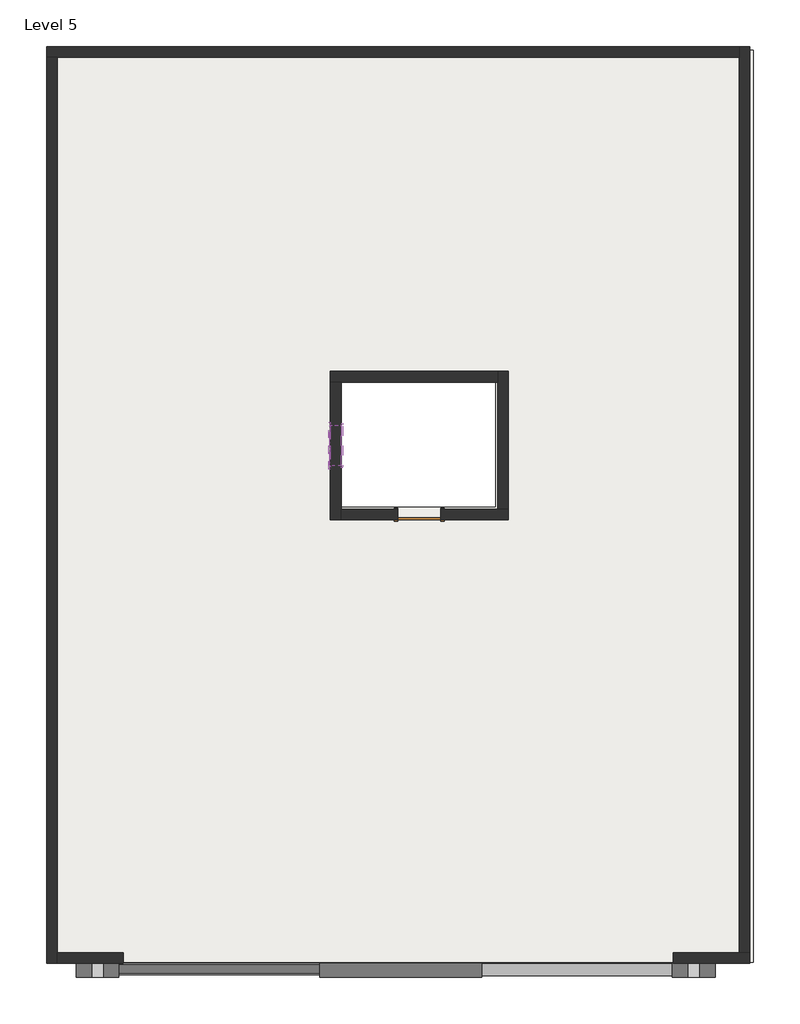
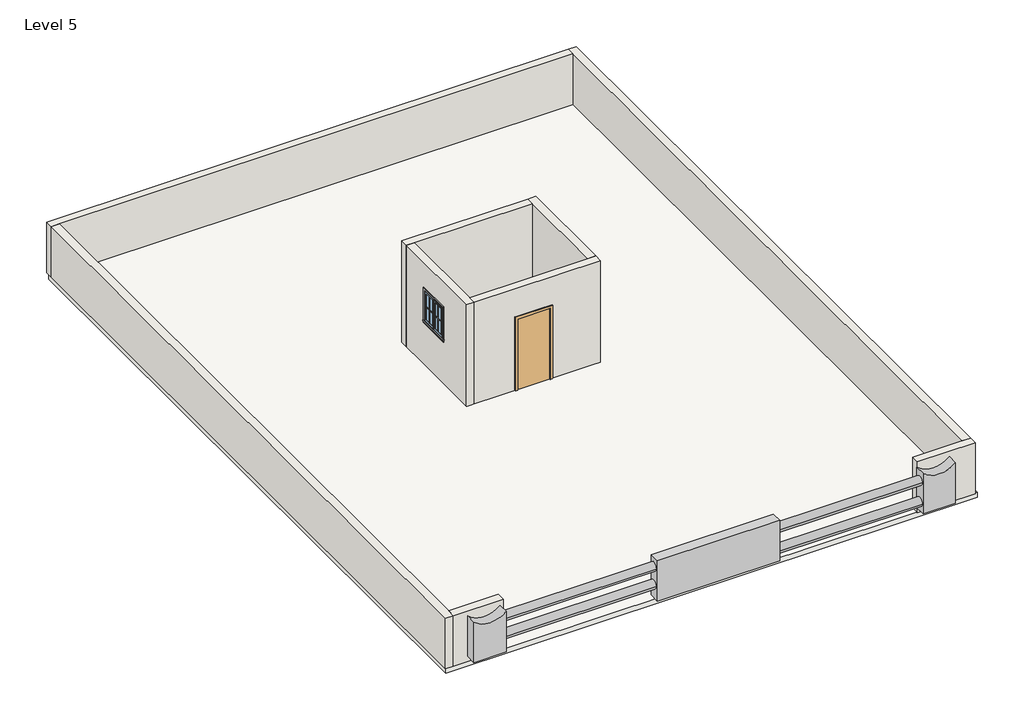
# One storey, incomplete: 9 walls, 8 proxies, 1 door, 1 roof, 1 window.
"""IFC4 building model written with IfcOpenShell, lengths in millimetres."""

from ifc_helpers import new_model, si_unit, frame, origin, place, context, project, spatial, polyline, outline, extrude, faceted_brep, transform, mapped, element, save
from components import generic_models_3_generic_models_3_b11e1288, generic_models_4_generic_models_4_816b7f5e, generic_models_5_generic_models_5_fbc28709, generic_models_6_generic_models_6_15436f46, muntin_pattern_2x2_muntin_pattern_2x2_b3fe6957, muntin_pattern_2x2_muntin_pattern_2x2_3e0ecaf2, trim_window_exterior_flat_with_sill_41619996, trim_window_interior_flat_picture_frame_51c85655, door_0ca8825f, window_339605e1

model = new_model("IFC4")

# Units and contexts
model_context = context("Model", 3, world=origin())
ifc_project = project(units=[si_unit("LENGTHUNIT", "METRE", prefix="MILLI")], contexts=[model_context])

# Site, building, storey
site = spatial("IfcSite", under=ifc_project)
building = spatial("IfcBuilding", under=site)
storey = spatial("IfcBuildingStorey", under=building, Name="Level 5", Elevation=9601.2)

# Proxies
placement = place(None, origin())
generic_models_3_generic_models_3_shape = generic_models_3_generic_models_3_b11e1288(model_context)
element("IfcBuildingElementProxy", 1, Name="Generic Models 3 : Generic Models 3", ObjectType="Generic Models 3 : Generic Models 3", at=placement, inside=storey, context=model_context, shape_type="MappedRepresentation", body=[
    mapped(generic_models_3_generic_models_3_shape, transform((0.0, 0.0, 0.0), x_axis=(1.0, 0.0, 0.0), y_axis=(0.0, 1.0, 0.0), z_axis=(0.0, 0.0, 1.0))),
])
generic_models_4_generic_models_4_shape = generic_models_4_generic_models_4_816b7f5e(model_context)
element("IfcBuildingElementProxy", 2, Name="Generic Models 4 : Generic Models 4", ObjectType="Generic Models 4 : Generic Models 4", at=placement, inside=storey, context=model_context, shape_type="MappedRepresentation", body=[
    mapped(generic_models_4_generic_models_4_shape, transform((0.0, 0.0, 0.0), x_axis=(1.0, 0.0, 0.0), y_axis=(0.0, 1.0, 0.0), z_axis=(0.0, 0.0, 1.0))),
])
generic_models_5_generic_models_5_shape = generic_models_5_generic_models_5_fbc28709(model_context)
element("IfcBuildingElementProxy", 3, Name="Generic Models 5 : Generic Models 5", ObjectType="Generic Models 5 : Generic Models 5", at=placement, inside=storey, context=model_context, shape_type="MappedRepresentation", body=[
    mapped(generic_models_5_generic_models_5_shape, transform((0.0, 0.0, 0.0), x_axis=(1.0, 0.0, 0.0), y_axis=(0.0, 1.0, 0.0), z_axis=(0.0, 0.0, 1.0))),
])
generic_models_6_generic_models_6_shape = generic_models_6_generic_models_6_15436f46(model_context)
element("IfcBuildingElementProxy", 4, Name="Generic Models 6 : Generic Models 6", ObjectType="Generic Models 6 : Generic Models 6", at=placement, inside=storey, context=model_context, shape_type="MappedRepresentation", body=[
    mapped(generic_models_6_generic_models_6_shape, transform((0.0, 0.0, 0.0), x_axis=(1.0, 0.0, 0.0), y_axis=(0.0, 1.0, 0.0), z_axis=(0.0, 0.0, 1.0))),
])
muntin_pattern_2x2_muntin_pattern_2x2_shape = muntin_pattern_2x2_muntin_pattern_2x2_b3fe6957(model_context)
element("IfcBuildingElementProxy", 5, Name="Muntin Pattern_2x2 : Muntin Pattern_2x2", ObjectType="Muntin Pattern_2x2 : Muntin Pattern_2x2", at=placement, inside=storey, context=model_context, shape_type="MappedRepresentation", body=[
    mapped(muntin_pattern_2x2_muntin_pattern_2x2_shape, transform((-2057.989408, 2363.8712675, 11020.6018488), x_axis=(0.0, 1.0, 0.0), y_axis=(-1.0, 0.0, 0.0), z_axis=(0.0, 0.0, 1.0))),
])
muntin_pattern_2x2_muntin_pattern_2x2_2_shape = muntin_pattern_2x2_muntin_pattern_2x2_3e0ecaf2(model_context)
element("IfcBuildingElementProxy", 6, Name="Muntin Pattern_2x2 : Muntin Pattern_2x2", ObjectType="Muntin Pattern_2x2 : Muntin Pattern_2x2", at=placement, inside=storey, context=model_context, shape_type="MappedRepresentation", body=[
    mapped(muntin_pattern_2x2_muntin_pattern_2x2_2_shape, transform((-2057.989408, 2792.4962675, 11020.6018488), x_axis=(0.0, -1.0, 0.0), y_axis=(1.0, 0.0, 0.0), z_axis=(0.0, 0.0, 1.0))),
])
trim_window_exterior_flat_with_sill_shape = trim_window_exterior_flat_with_sill_41619996(model_context)
element("IfcBuildingElementProxy", 7, Name="Trim-Window-Exterior-Flat : with Sill", ObjectType="Trim-Window-Exterior-Flat : with Sill", at=placement, inside=storey, context=model_context, shape_type="MappedRepresentation", body=[
    mapped(trim_window_exterior_flat_with_sill_shape, transform((-2067.514408, 2578.1837675, 11865.1518488), x_axis=(0.0, -1.0, 0.0), y_axis=(0.0, 0.0, 1.0), z_axis=(-1.0, 0.0, 0.0))),
])
trim_window_interior_flat_picture_frame_shape = trim_window_interior_flat_picture_frame_51c85655(model_context)
element("IfcBuildingElementProxy", 8, Name="Trim-Window-Interior-Flat : Picture Frame", ObjectType="Trim-Window-Interior-Flat : Picture Frame", at=placement, inside=storey, context=model_context, shape_type="MappedRepresentation", body=[
    mapped(trim_window_interior_flat_picture_frame_shape, transform((-1838.914408, 2578.1837675, 11865.1518488), x_axis=(0.0, 1.0, 0.0), y_axis=(0.0, 0.0, 1.0), z_axis=(1.0, 0.0, 0.0))),
])

# Door
door_shape = door_0ca8825f(model_context)
element("IfcDoor", 9, ObjectType="Single-Flush : 36\" x 84\"", at=placement, inside=storey, context=model_context, shape_type="MappedRepresentation", body=[
    mapped(door_shape, transform((-165.9529582, 1103.8652728, 9601.2), x_axis=(-1.0, 0.0, 0.0), y_axis=(0.0, -1.0, 0.0), z_axis=(0.0, 0.0, 1.0))),
])

# Roof
element("IfcRoof", 10, ObjectType="Generic - 12\"", at=placement, inside=storey, context=model_context, shape_type="SweptSolid", body=[
    extrude(outline(polyline([(-8113.2415084, -8469.6977377), (-8113.2415084, 11037.5022623), (6974.3584916, 11037.5022623), (6974.3584916, -8469.6977377), (-8113.2415084, -8469.6977377)]), holes=[polyline([(1456.2084916, 3938.2022623), (-1838.914408, 3938.2022623), (-1838.914408, 1268.9652728), (1456.2084916, 1268.9652728), (1456.2084916, 3938.2022623)])]), frame((0.0, 0.0, 9448.8), z_axis=(0.0, 0.0, 1.0), x_axis=(1.0, 0.0, 0.0)), (0.0, 0.0, 1.0), 152.4),
])

# Walls
element("IfcWall", 11, ObjectType="9\"", at=placement, inside=storey, context=model_context, shape_type="Brep", body=[
    faceted_brep([(-8138.6415084, 10885.1022623, 9601.2), (-7910.0415084, 10885.1022623, 9601.2), (6669.5584916, 10885.1022623, 9601.2), (6669.5584916, 10885.1022623, 11125.2), (-7910.0415084, 10885.1022623, 11125.2), (-8138.6415084, 10885.1022623, 11125.2), (-8138.6415084, 11113.7022623, 9601.2), (-8138.6415084, 11113.7022623, 11125.2), (6669.5584916, 11113.7022623, 11125.2), (6669.5584916, 11113.7022623, 9601.2)], [[[0, 1, 2, 3, 4, 5]], [[6, 7, 8, 9]], [[2, 1, 0, 6, 9]], [[5, 4, 3, 8, 7]], [[0, 5, 7, 6]], [[3, 2, 9, 8]]]),
])
element("IfcWall", 12, ObjectType="9\"", at=placement, inside=storey, context=model_context, shape_type="Brep", body=[
    faceted_brep([(-7910.0415084, -8488.7477377, 9601.2), (-7910.0415084, -8260.1477377, 9601.2), (-7910.0415084, 10885.1022623, 9601.2), (-7910.0415084, 10885.1022623, 11125.2), (-7910.0415084, -8260.1477377, 11125.2), (-7910.0415084, -8488.7477377, 11125.2), (-8138.6415084, -8488.7477377, 9601.2), (-8138.6415084, -8488.7477377, 11125.2), (-8138.6415084, 10885.1022623, 11125.2), (-8138.6415084, 10885.1022623, 9601.2)], [[[0, 1, 2, 3, 4, 5]], [[6, 7, 8, 9]], [[2, 1, 0, 6, 9]], [[5, 4, 3, 8, 7]], [[0, 5, 7, 6]], [[3, 2, 9, 8]]]),
])
element("IfcWall", 13, ObjectType="9\"", at=placement, inside=storey, context=model_context, shape_type="Brep", body=[
    faceted_brep([(6898.1584916, -8260.1477377, 9601.2), (6669.5584916, -8260.1477377, 9601.2), (5259.8584916, -8260.1477377, 9601.2), (5259.8584916, -8260.1477377, 11125.2), (6669.5584916, -8260.1477377, 11125.2), (6898.1584916, -8260.1477377, 11125.2), (6898.1584916, -8488.7477377, 9601.2), (6898.1584916, -8488.7477377, 11125.2), (5259.8584916, -8488.7477377, 11125.2), (5259.8584916, -8488.7477377, 9601.2)], [[[0, 1, 2, 3, 4, 5]], [[6, 7, 8, 9]], [[2, 1, 0, 6, 9]], [[3, 2, 9, 8]], [[5, 4, 3, 8, 7]], [[0, 5, 7, 6]]]),
])
element("IfcWall", 14, ObjectType="9\"", at=placement, inside=storey, context=model_context, shape_type="Brep", body=[
    faceted_brep([(6669.5584916, 11113.7022623, 9601.2), (6669.5584916, 10885.1022623, 9601.2), (6669.5584916, -8260.1477377, 9601.2), (6669.5584916, -8260.1477377, 11125.2), (6669.5584916, 10885.1022623, 11125.2), (6669.5584916, 11113.7022623, 11125.2), (6898.1584916, 11113.7022623, 9601.2), (6898.1584916, 11113.7022623, 11125.2), (6898.1584916, -8260.1477377, 11125.2), (6898.1584916, -8260.1477377, 9601.2)], [[[0, 1, 2, 3, 4, 5]], [[6, 7, 8, 9]], [[2, 1, 0, 6, 9]], [[5, 4, 3, 8, 7]], [[0, 5, 7, 6]], [[3, 2, 9, 8]]]),
])
element("IfcWall", 15, ObjectType="9\"", at=placement, inside=storey, context=model_context, shape_type="Brep", body=[
    faceted_brep([(-2067.514408, 3938.2022623, 9601.2), (-1838.914408, 3938.2022623, 9601.2), (1507.0084916, 3938.2022623, 9601.2), (1507.0084916, 3938.2022623, 12649.2), (-1838.914408, 3938.2022623, 12649.2), (-2067.514408, 3938.2022623, 12649.2), (-2067.514408, 4166.8022623, 9601.2), (-2067.514408, 4166.8022623, 12649.2), (1507.0084916, 4166.8022623, 12649.2), (1507.0084916, 4166.8022623, 9601.2)], [[[0, 1, 2, 3, 4, 5]], [[6, 7, 8, 9]], [[2, 1, 0, 6, 9]], [[5, 4, 3, 8, 7]], [[0, 5, 7, 6]], [[3, 2, 9, 8]]]),
])
element("IfcWall", 16, ObjectType="9\"", at=placement, inside=storey, context=model_context, shape_type="Brep", body=[
    faceted_brep([(-1838.914408, 989.5652728, 9601.2), (-1838.914408, 1218.1652728, 9601.2), (-1838.914408, 3938.2022623, 9601.2), (-1838.914408, 3938.2022623, 12649.2), (-1838.914408, 1218.1652728, 12649.2), (-1838.914408, 989.5652728, 12649.2), (-1838.914408, 3009.9837675, 11865.1518488), (-1838.914408, 3009.9837675, 10950.7518488), (-1838.914408, 2146.3837675, 10950.7518488), (-1838.914408, 2146.3837675, 11865.1518488), (-2067.514408, 989.5652728, 9601.2), (-2067.514408, 989.5652728, 12649.2), (-2067.514408, 3938.2022623, 12649.2), (-2067.514408, 3938.2022623, 9601.2), (-2067.514408, 3009.9837675, 11865.1518488), (-2067.514408, 2146.3837675, 11865.1518488), (-2067.514408, 2146.3837675, 10950.7518488), (-2067.514408, 3009.9837675, 10950.7518488)], [[[0, 1, 2, 3, 4, 5], [6, 7, 8, 9]], [[10, 11, 12, 13], [14, 15, 16, 17]], [[2, 1, 0, 10, 13]], [[5, 4, 3, 12, 11]], [[0, 5, 11, 10]], [[3, 2, 13, 12]], [[7, 6, 14, 17]], [[8, 7, 17, 16]], [[9, 8, 16, 15]], [[6, 9, 15, 14]]]),
])
element("IfcWall", 17, ObjectType="9\"", at=placement, inside=storey, context=model_context, shape_type="Brep", body=[
    faceted_brep([(-623.1529582, 1218.1652728, 11734.8), (-623.1529582, 1218.1652728, 9601.2), (-1838.914408, 1218.1652728, 9601.2), (-1838.914408, 1218.1652728, 12649.2), (1507.0084916, 1218.1652728, 12649.2), (1735.6084916, 1218.1652728, 12649.2), (1735.6084916, 1218.1652728, 9601.2), (1507.0084916, 1218.1652728, 9601.2), (291.2470418, 1218.1652728, 9601.2), (291.2470418, 1218.1652728, 11734.8), (-1838.914408, 989.5652728, 9601.2), (-623.1529582, 989.5652728, 9601.2), (-623.1529582, 989.5652728, 11734.8), (291.2470418, 989.5652728, 11734.8), (291.2470418, 989.5652728, 9601.2), (1735.6084916, 989.5652728, 9601.2), (1735.6084916, 989.5652728, 12649.2), (-1838.914408, 989.5652728, 12649.2)], [[[0, 1, 2, 3, 4, 5, 6, 7, 8, 9]], [[10, 11, 12, 13, 14, 15, 16, 17]], [[2, 1, 11, 10]], [[8, 7, 6, 15, 14]], [[5, 4, 3, 17, 16]], [[6, 5, 16, 15]], [[3, 2, 10, 17]], [[12, 11, 1, 0]], [[13, 12, 0, 9]], [[14, 13, 9, 8]]]),
])
element("IfcWall", 18, ObjectType="9\"", at=placement, inside=storey, context=model_context, shape_type="Brep", body=[
    faceted_brep([(1507.0084916, 4166.8022623, 9601.2), (1507.0084916, 3938.2022623, 9601.2), (1507.0084916, 1218.1652728, 9601.2), (1507.0084916, 1218.1652728, 12649.2), (1507.0084916, 3938.2022623, 12649.2), (1507.0084916, 4166.8022623, 12649.2), (1735.6084916, 4166.8022623, 9601.2), (1735.6084916, 4166.8022623, 12649.2), (1735.6084916, 1218.1652728, 12649.2), (1735.6084916, 1218.1652728, 9601.2)], [[[0, 1, 2, 3, 4, 5]], [[6, 7, 8, 9]], [[2, 1, 0, 6, 9]], [[5, 4, 3, 8, 7]], [[0, 5, 7, 6]], [[3, 2, 9, 8]]]),
])
element("IfcWall", 19, ObjectType="9\"", at=placement, inside=storey, context=model_context, shape_type="SweptSolid", body=[
    extrude(outline(polyline([(-7910.0415084, -8260.1477377), (-6500.3415084, -8260.1477377), (-6500.3415084, -8488.7477377), (-7910.0415084, -8488.7477377), (-7910.0415084, -8260.1477377)])), frame((0.0, 0.0, 9601.2), z_axis=(0.0, 0.0, 1.0), x_axis=(1.0, 0.0, 0.0)), (0.0, 0.0, 1.0), 1524.0),
])

# Window
window_shape = window_339605e1(model_context)
element("IfcWindow", 20, ObjectType="Window-Casement-Double : 34\" x 36\"", at=placement, inside=storey, context=model_context, shape_type="MappedRepresentation", body=[
    mapped(window_shape, transform((-1953.214408, 2578.1837675, 10036.3518488), x_axis=(0.0, 1.0, 0.0), y_axis=(-1.0, 0.0, 0.0), z_axis=(0.0, 0.0, 1.0))),
])

save(model, "model.ifc")

# Revit data of these elements
# Type "Muntin Pattern_2x2 : Muntin Pattern_2x2"
#   Width [instance default] = 4' - 0"
#   Thickness = 0' - 0 1/2"
#   Height [instance default] = 4' - 0"
#   Distance = 0' - 0 3/4"
#   Interior Material [instance default] = none
#   Exterior Material [instance default] = none
#   Default Elevation = 0
# Type "Trim-Window-Exterior-Flat : with Sill"
#   Trim Width = 0' - 2 1/4"
#   Trim Thickness_Picture Frame = 0' - 1 1/4"
#   Trim Thickness_with Sill = 0' - 0 3/4"
#   Sill Thickness = 0' - 1 1/4"
#   Opening Width [instance default] = 2' - 0"
#   Opening Height [instance default] = 3' - 0"
#   Default Elevation = 4' - 0"
#   Sill = yes
#   Picture Frame = no
#   Trim Material [instance default] = none
# Type "Trim-Window-Interior-Flat : Picture Frame"
#   Trim Thickness_Picture Frame = 0' - 1 1/4"
#   Trim Width = 0' - 2 1/4"
#   Trim Thickness_with Sill = 0' - 0 3/4"
#   Sill Thickness = 0' - 1 1/4"
#   Opening Width [instance default] = 2' - 0"
#   Opening Height [instance default] = 3' - 0"
#   Default Elevation = 4' - 0"
#   Sill = no
#   Picture Frame = yes
#   Trim Material [instance default] = none
# Type "Single-Flush : 36\" x 84\""
#   Type Mark = "1"
#   Construction Type Id = "MDOOR"
#   Assembly Code = "C1020"
#   Analytic Construction = "Metal"
#   Thickness = 0' - 2"
#   Heat Transfer Coefficient (U) = 0.651978 BTU/(h·ft²·°F)
#   Height = 7' - 0"
#   Trim Projection Ext = 0' - 1"
#   Trim Projection Int = 0' - 1"
#   Trim Width = 0' - 3"
#   Width = 3' - 0"
#   Define Thermal Properties by = 1
#   Define Thermal Properties by = 1
#   Door Material = Door - Panel
#   Frame Material = Door - Frame
#   Visual Light Transmittance = 0
#   Solar Heat Gain Coefficient = 0
#   Function = (empty or 0)
#   Wall Closure = (empty or 0)
# Type "Generic - 12\""
#   Assembly Code = "B1020"
#   Layers, outside or top first: 0' - 6" no material (function 1)
# Type "9\""
#   Assembly Code = "B2010"
#   Layers, outside or top first: 0' - 9" no material (function 1)
# Type "Window-Casement-Double : 34\" x 36\""
#   Type Mark = "14"
#   Fire Rating = "0.5h"
#   Assembly Code = "B2020100"
#   Analytic Construction = "Double glazing - domestic"
#   Frame Extension [instance default] = 0' - 0 1/4"
#   Window Inset [instance default] = 0' - 0"
#   Wall Thickness [instance default] = 0' - 6"
#   Interior Wall Closure [instance default] = 0' - 2 1/4"
#   Half Width = 1' - 5"
#   Visual Light Transmittance = 0.81
#   Thermal Resistance (R) = 1.8146 (h·ft²·°F)/BTU
#   Solar Heat Gain Coefficient = 0.76
#   Rough Width = 2' - 10 1/2"
#   Rough Height = 3' - 0 1/2"
#   Height = 3' - 0"
#   Heat Transfer Coefficient (U) = 0.5511 BTU/(h·ft²·°F)
#   Exterior Wall Closure [instance default] = 0' - 1 1/4"
#   Extension Jamb [instance default] = 0' - 2 1/4"
#   Default Sill Height = 3' - 0"
#   Width = 2' - 10"
#   Define Thermal Properties by = 0
#   Muntin Visibility = yes
#   Interior Trim Visibility [instance default] = yes
#   Exterior Trim Visibility [instance default] = yes
#   Extension Jamb Visibility [instance default] = yes
#   Interior Trim Material = Wood - Stained
#   Muntin Pattern = Muntin Pattern_2x2 : Muntin Pattern_2x2
#   Interior Trim = Trim-Window-Interior-Flat : Picture Frame
#   Interior Frame Material = Wood - Stained
#   Glass Panel Material = Glass
#   Exterior Trim Material = Clad - White
#   Exterior Trim = Trim-Window-Exterior-Flat : with Sill
#   Exterior Frame Material = Clad - White
#   Wall Closure = (empty or 0)
# Element 1 (IfcBuildingElementProxy, "Generic Models 3 : Generic Models 3")
#   Phase Created = New Construction
#   Materials on its faces: "Door - Frame"
# Element 2 (IfcBuildingElementProxy, "Generic Models 4 : Generic Models 4")
#   Phase Created = New Construction
#   Materials on its faces: "Brick, Soldier Course"
# Element 3 (IfcBuildingElementProxy, "Generic Models 5 : Generic Models 5")
#   Phase Created = New Construction
#   Materials on its faces: "Parking Stripe"
# Element 4 (IfcBuildingElementProxy, "Generic Models 6 : Generic Models 6")
#   Phase Created = New Construction
#   Materials on its faces: "Brick, Soldier Course"
# Elements 5, 6 (IfcBuildingElementProxy, "Muntin Pattern_2x2 : Muntin Pattern_2x2")
#   Width = 0' - 11 5/8"
#   Height = 2' - 6 1/2"
#   Interior Material = Wood - Stained
#   Exterior Material = Clad - White
#   Phase Created = New Construction
#   Materials on its faces: "Clad - White", "Wood - Stained"
# Element 7 (IfcBuildingElementProxy, "Trim-Window-Exterior-Flat : with Sill")
#   Opening Width = 2' - 10"
#   Opening Height = 3' - 0"
#   Trim Material = Clad - White
#   Phase Created = New Construction
#   Materials on its faces: "Clad - White"
# Element 8 (IfcBuildingElementProxy, "Trim-Window-Interior-Flat : Picture Frame")
#   Opening Width = 2' - 10"
#   Opening Height = 3' - 0"
#   Trim Material = Wood - Stained
#   Phase Created = New Construction
#   Materials on its faces: "Wood - Stained"
# Element 9 (IfcDoor, "Single-Flush : 36\" x 84\"")
#   Phase Created = New Construction
#   Materials on its faces: "Door - Frame", "Door - Panel"
# Element 10 (IfcRoof, "Generic - 12\"")
#   built-in parameter 1001705 = 31.5 (stored number, unit not read)
#   built-in parameter 1001701 = -0.5 (stored number, unit not read)
#   built-in parameter 1001710 = 33615
#   Phase Created = New Construction
#   Materials on its faces: "Default Roof"
# Elements 11, 12, 14 (IfcWall, "9\"")
#   Top Offset = 0' - 0"
#   Base Offset = 0' - 0"
#   Unconnected Height = 5' - 0"
#   wall height = 5' - 0"
#   Phase Created = New Construction
#   Base Constraint = Level 5
#   Materials on its faces: "Blanket", "Default Wall"
# Element 13 (IfcWall, "9\"")
#   Top Offset = 0' - 0"
#   Base Offset = 0' - 0"
#   Unconnected Height = 5' - 0"
#   wall height = 5' - 0"
#   Phase Created = New Construction
#   Base Constraint = Level 5
#   Materials on its faces: "Default Wall", "Blanket", "Carpet (1)"
# Elements 15, 16, 18 (IfcWall, "9\"")
#   Top Offset = 0' - 0"
#   Base Offset = 0' - 0"
#   Unconnected Height = 10' - 0"
#   wall height = 10' - 0"
#   Phase Created = New Construction
#   Base Constraint = Level 5
#   Materials on its faces: "Default Wall", "Wood - Stained"
# Element 17 (IfcWall, "9\"")
#   Top Offset = 0' - 0"
#   Base Offset = 0' - 0"
#   Unconnected Height = 10' - 0"
#   wall height = 10' - 0"
#   Phase Created = New Construction
#   Base Constraint = Level 5
#   Materials on its faces: "Default Wall", "legs", "Wood - Stained"
# Element 19 (IfcWall, "9\"")
#   Top Offset = 0' - 0"
#   Base Offset = 0' - 0"
#   Unconnected Height = 5' - 0"
#   wall height = 5' - 0"
#   Phase Created = New Construction
#   Base Constraint = Level 5
#   Materials on its faces: "Default Wall", "Carpet (1)", "Blanket"
# Element 20 (IfcWindow, "Window-Casement-Double : 34\" x 36\"")
#   Mark = "31"
#   Window Inset = 0' - 0"
#   Interior Wall Closure = 0' - 2 1/4"
#   Frame Extension = 0' - 0 1/4"
#   Exterior Wall Closure = 0' - 1 1/4"
#   Interior Trim Visibility = yes
#   Exterior Trim Visibility = yes
#   Phase Created = New Construction
#   Materials on its faces: "Wood - Stained", "Glass", "Clad - White"
# Materials
#   "Door - Panel": class "Wood", colour RGB 210 159 95, transparency 0, Cost = 0
#   "Door - Frame": colour RGB 118 70 51, transparency 0, Cost = 0
#   "Wood - Stained": class "Wood", colour RGB 224 178 126, transparency 0, Cost = 0
#   "Glass": class "Glass", colour RGB 0 128 192, transparency 0.75, Description = "Soda Lime Glass", Cost = 0
#   "Clad - White": class "Wood", colour RGB 242 242 238, transparency 0, Cost = 0
#   "Brick, Soldier Course": class "Masonry", colour RGB 170 98 104, transparency 0, Description = "Common brick soldier coursed", Cost = 0
#   "Parking Stripe": class "Paint", colour RGB 250 250 91, transparency 0, Cost = 0
#   "Default Roof": colour RGB 88 101 114, transparency 0, Cost = 0
#   "Blanket": class "System", colour RGB 59 0 1, transparency 0, Cost = 0
#   "Default Wall": colour RGB 128 128 128, transparency 0, Cost = 0
#   "Carpet (1)": class "Carpet", colour RGB 124 80 67, transparency 0, Description = "Interior finish", Cost = 0
#   "legs": colour RGB 90 73 37, transparency 0, Cost = 0
